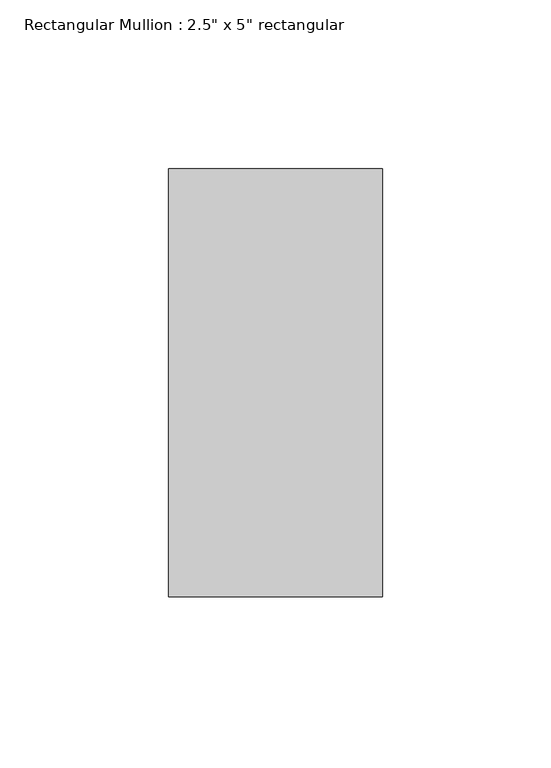
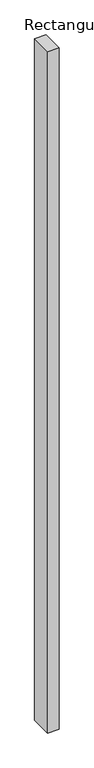
"""IFC4 building model written with IfcOpenShell, lengths in millimetres: member geometry."""

from ifc_helpers import new_model, si_unit, frame, origin, place, context, project, spatial, polyline, outline, extrude, source, transform, mapped, element, save


def member_6f9d7b88(model_context):
    return source(origin(), model_context, "Body", "SweptSolid", [
        extrude(outline(polyline([(0.0, 63.5), (0.0, -63.5), (-63.5, -63.5), (-63.5, 63.5), (0.0, 63.5)])), frame((0.0, 0.0, -4064.0), z_axis=(0.0, 0.0, 1.0), x_axis=(1.0, 0.0, 0.0)), (0.0, 0.0, 1.0), 4064.0),
    ])


if __name__ == "__main__":
    model = new_model("IFC4")
    model_context = context("Model", 3, world=origin())
    ifc_project = project(units=[si_unit("LENGTHUNIT", "METRE", prefix="MILLI")], contexts=[model_context])
    site = spatial("IfcSite", under=ifc_project)
    building = spatial("IfcBuilding", under=site)
    placement = place(None, origin())
    member_shape = member_6f9d7b88(model_context)
    element("IfcMember", 1, ObjectType="Rectangular Mullion : 2.5\" x 5\" rectangular", at=placement, inside=building, context=model_context, shape_type="MappedRepresentation", body=[
        mapped(member_shape, transform((0.0, 0.0, 0.0), x_axis=(1.0, 0.0, 0.0), y_axis=(0.0, 1.0, 0.0), z_axis=(0.0, 0.0, 1.0))),
    ])
    save(model, "model.ifc")

# Revit data of these elements
# Type "Rectangular Mullion : 2.5\" x 5\" rectangular"
#   built-in parameter 1007304 = 0.416667 (stored number, unit not read)
#   built-in parameter 1007301 = 0.104167 (stored number, unit not read)
#   built-in parameter 1007300 = 0.104167 (stored number, unit not read)
# Element 1 (IfcMember, "Rectangular Mullion : 2.5\" x 5\" rectangular")
#   Materials on its faces: "Aluminum"
# Materials
#   "Aluminum": class "Metal", colour RGB 247 247 247, transparency 0, Description = "Aluminum 6061", Cost = 0
